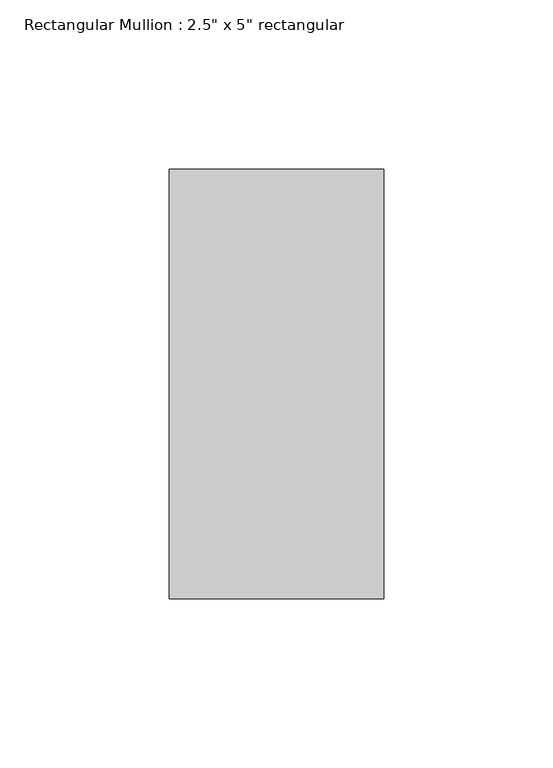
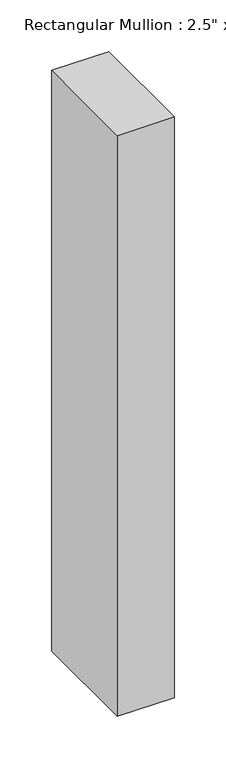
"""IFC4 building model written with IfcOpenShell, lengths in millimetres: member geometry."""

from ifc_helpers import new_model, si_unit, frame, origin, place, context, project, spatial, polyline, outline, extrude, source, transform, mapped, element, save


def member_6e28d7e1(model_context):
    return source(origin(), model_context, "Body", "SweptSolid", [
        extrude(outline(polyline([(0.0, 63.5), (0.0, -63.5), (-63.5, -63.5), (-63.5, 63.5), (0.0, 63.5)])), frame((0.0, 0.0, -685.8), z_axis=(0.0, 0.0, 1.0), x_axis=(1.0, 0.0, 0.0)), (0.0, 0.0, 1.0), 685.8),
    ])


if __name__ == "__main__":
    model = new_model("IFC4")
    model_context = context("Model", 3, world=origin())
    ifc_project = project(units=[si_unit("LENGTHUNIT", "METRE", prefix="MILLI")], contexts=[model_context])
    site = spatial("IfcSite", under=ifc_project)
    building = spatial("IfcBuilding", under=site)
    placement = place(None, origin())
    member_shape = member_6e28d7e1(model_context)
    element("IfcMember", 1, ObjectType="Rectangular Mullion : 2.5\" x 5\" rectangular", at=placement, inside=building, context=model_context, shape_type="MappedRepresentation", body=[
        mapped(member_shape, transform((0.0, 0.0, 0.0), x_axis=(1.0, 0.0, 0.0), y_axis=(0.0, 1.0, 0.0), z_axis=(0.0, 0.0, 1.0))),
    ])
    save(model, "model.ifc")

# Revit data of these elements
# Type "Rectangular Mullion : 2.5\" x 5\" rectangular"
#   built-in parameter 1007304 = 0.416667 (stored number, unit not read)
#   built-in parameter 1007301 = 0.104167 (stored number, unit not read)
#   built-in parameter 1007300 = 0.104167 (stored number, unit not read)
# Element 1 (IfcMember, "Rectangular Mullion : 2.5\" x 5\" rectangular")
#   Materials on its faces: "Aluminum"
# Materials
#   "Aluminum": class "Metal", colour RGB 247 247 247, transparency 0, Description = "Aluminum 6061", Cost = 0
